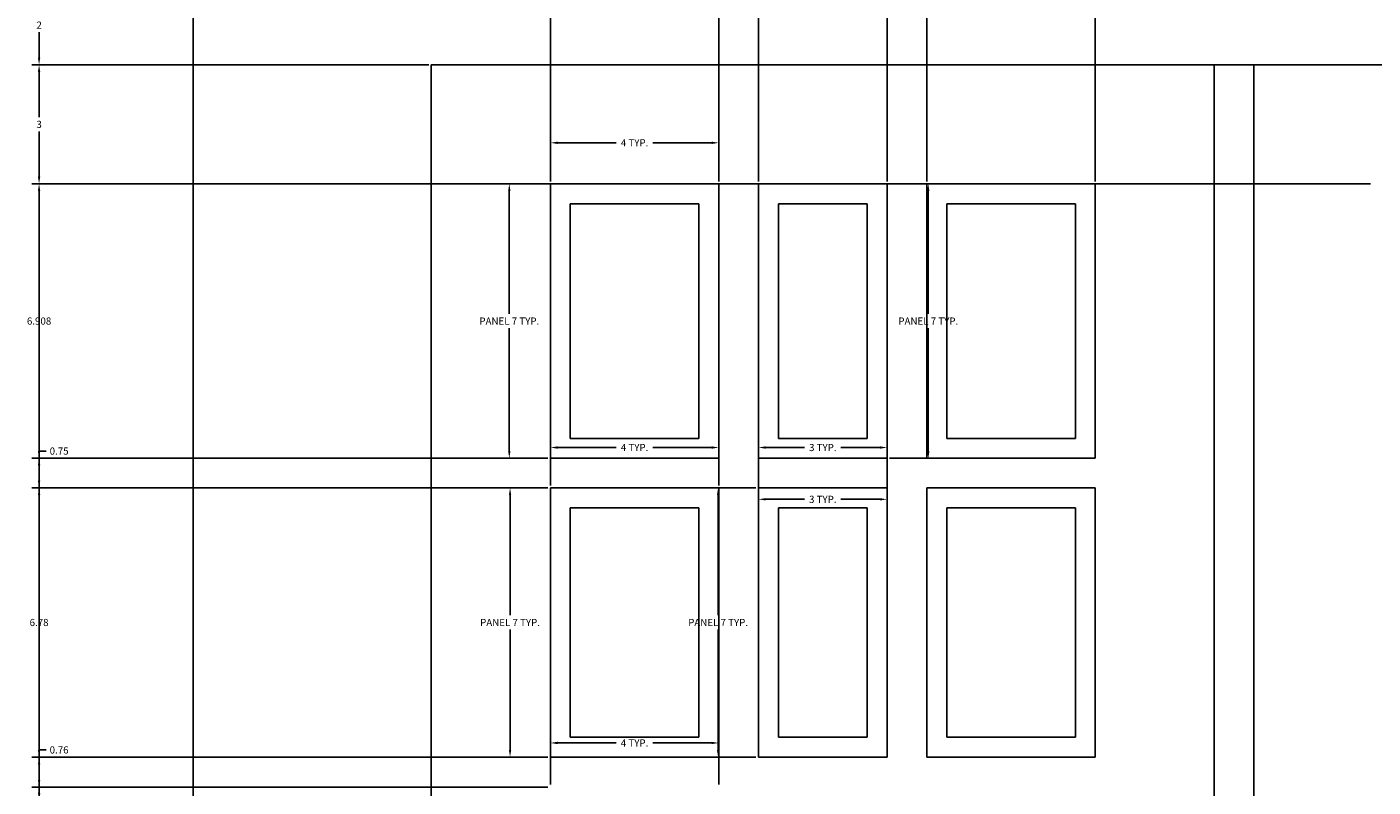
# Model space of a CAD drawing. Units: inches. Extents: x 12532.3 to 12594.9, y 6967.5 to 7063.
# Tile 3 of 9: x 12532.3 to 12566.2, y 7000.7 to 7019.9. Entities that reach past the tile are written whole.
import ezdxf

# ---------------------------------------------------------------- set-up
doc = ezdxf.new("R2010")
doc.units = ezdxf.units.IN
doc.header["$MEASUREMENT"] = 0
doc.header["$PDMODE"] = 98
doc.layers.add('A-ANNO-DIMS', color=2, linetype='Continuous', lineweight=18)
doc.layers.add('A-DOOR', color=4, linetype='Continuous', lineweight=25)
doc.styles.get("Standard").update_dxf_attribs({"font": 'arial.ttf'})
doc.dimstyles.get("Standard").update_dxf_attribs({"dimtxt": 0.18, "dimasz": 0.18, "dimexe": 0.18, "dimexo": 0.0625, "dimgap": 0.09, "dimtad": 0, "dimtih": 1, "dimtoh": 1, "dimdec": 4, "dimzin": 0, "dimdsep": 46, "dimtxsty": 'Standard', "dimcen": 0.09, "dimadec": 0, "dimazin": 0, "dimtfac": 1, "dimtdec": 4, "dimtofl": 0, "dimtmove": 0, "dimatfit": 3, "dimfxl": 1, "dimtolj": 1, "dimtzin": 0, "dimarcsym": 0})

# ---------------------------------------------------------------- blocks, each defined once
blk = doc.blocks.new('DOOR-PANEL-4_2x6_9')
for p, q in [((4.241, 6.908), (0, 6.908)), ((0, 6.908), (0, 0)), ((4.241, 6.908), (4.241, 0)), ((3.741, 6.408), (0.5, 6.408)), ((0.5, 6.408), (0.5, 0.5)), ((3.741, 6.408), (3.741, 0.5)), ((3.741, 0.5), (0.5, 0.5)), ((4.241, 0), (0, 0))]:
    blk.add_line(p, q)
blk = doc.blocks.new('DOOR-PANEL-4_2x6_8')
for p, q in [((4.241, 6.78), (0, 6.78)), ((0, 6.78), (0, 0)), ((4.241, 6.78), (4.241, 0)), ((3.741, 6.28), (0.5, 6.28)), ((0.5, 6.28), (0.5, 0.5)), ((3.741, 6.28), (3.741, 0.5)), ((3.741, 0.5), (0.5, 0.5)), ((4.241, 0), (0, 0))]:
    blk.add_line(p, q)
blk = doc.blocks.new('DOOR-PANEL-3_2x6_8')
for p, q in [((0, 6.78), (0, 0)), ((3.24, 6.78), (0, 6.78)), ((3.24, 6.78), (3.24, 0)), ((0.5, 6.28), (0.5, 0.5)), ((2.74, 6.28), (0.5, 6.28)), ((2.74, 6.28), (2.74, 0.5)), ((2.74, 0.5), (0.5, 0.5)), ((3.24, 0), (0, 0))]:
    blk.add_line(p, q)
blk = doc.blocks.new('DOOR-PANEL-3_2x6_9')
for p, q in [((0, 0), (0, 6.908)), ((0, 6.908), (3.24, 6.908)), ((3.24, 0), (3.24, 6.908)), ((0.5, 0.5), (0.5, 6.408)), ((0.5, 6.408), (2.74, 6.408)), ((2.74, 0.5), (2.74, 6.408)), ((0.5, 0.5), (2.74, 0.5)), ((0, 0), (3.24, 0))]:
    blk.add_line(p, q)
blk = doc.blocks.new('*D13')
at = {"layer": 'A-ANNO-DIMS', "color": 0, "lineweight": -2, "transparency": 16777216}
for p, q in [((12545.388, 7015.929), (12544.234, 7015.929)), ((12544.414, 7015.749), (12544.414, 7012.655)), ((12544.414, 7009.201), (12544.414, 7012.295)), ((12545.388, 7009.021), (12544.234, 7009.021))]:
    blk.add_line(p, q, dxfattribs=at)
at = {"layer": 'A-ANNO-DIMS', "color": 0, "transparency": 16777216}
for points in [[(12544.384, 7015.749), (12544.444, 7015.749), (12544.414, 7015.929)], [(12544.384, 7009.201), (12544.444, 7009.201), (12544.414, 7009.021)]]:
    blk.add_solid(points, dxfattribs=at)
at = {"layer": 'Defpoints', "color": 0, "transparency": 16777216}
for p in [(12545.45, 7015.929), (12544.414, 7009.021), (12545.45, 7009.021)]:
    blk.add_point(p, dxfattribs=at)
at = {"layer": 'A-ANNO-DIMS', "color": 0, "transparency": 16777216, "insert": (12544.414, 7012.475), "char_height": 0.18, "attachment_point": 5}
blk.add_mtext('\\A1;PANEL 7 TYP.', dxfattribs=at)
blk = doc.blocks.new('*D14')
at = {"layer": 'A-ANNO-DIMS', "color": 0, "lineweight": -2, "transparency": 16777216}
for p, q in [((12545.45, 7015.991), (12545.45, 7017.145)), ((12549.691, 7015.991), (12549.691, 7017.145)), ((12545.63, 7016.965), (12547.109, 7016.965)), ((12549.511, 7016.965), (12548.032, 7016.965))]:
    blk.add_line(p, q, dxfattribs=at)
at = {"layer": 'A-ANNO-DIMS', "color": 0, "transparency": 16777216}
for points in [[(12545.63, 7016.995), (12545.63, 7016.935), (12545.45, 7016.965)], [(12549.511, 7016.995), (12549.511, 7016.935), (12549.691, 7016.965)]]:
    blk.add_solid(points, dxfattribs=at)
at = {"layer": 'Defpoints', "color": 0, "transparency": 16777216}
for p in [(12545.45, 7016.965), (12545.45, 7015.929), (12549.691, 7015.929)]:
    blk.add_point(p, dxfattribs=at)
at = {"layer": 'A-ANNO-DIMS', "color": 0, "transparency": 16777216, "insert": (12547.57, 7016.965), "char_height": 0.18, "attachment_point": 5}
blk.add_mtext('\\A1;4 TYP.', dxfattribs=at)
blk = doc.blocks.new('*D15')
at = {"layer": 'A-ANNO-DIMS', "color": 0, "lineweight": -2, "transparency": 16777216}
for p, q in [((12545.388, 7008.273), (12544.253, 7008.273)), ((12544.433, 7008.093), (12544.433, 7005.064)), ((12544.433, 7001.673), (12544.433, 7004.703)), ((12545.388, 7001.493), (12544.253, 7001.493))]:
    blk.add_line(p, q, dxfattribs=at)
at = {"layer": 'A-ANNO-DIMS', "color": 0, "transparency": 16777216}
for points in [[(12544.403, 7008.093), (12544.463, 7008.093), (12544.433, 7008.273)], [(12544.403, 7001.673), (12544.463, 7001.673), (12544.433, 7001.493)]]:
    blk.add_solid(points, dxfattribs=at)
at = {"layer": 'Defpoints', "color": 0, "transparency": 16777216}
for p in [(12545.45, 7008.273), (12544.433, 7001.493), (12545.45, 7001.493)]:
    blk.add_point(p, dxfattribs=at)
at = {"layer": 'A-ANNO-DIMS', "color": 0, "transparency": 16777216, "insert": (12544.433, 7004.883), "char_height": 0.18, "attachment_point": 5}
blk.add_mtext('\\A1;PANEL 7 TYP.', dxfattribs=at)
blk = doc.blocks.new('*D16')
at = {"layer": 'A-ANNO-DIMS', "color": 0, "lineweight": -2, "transparency": 16777216}
for p, q in [((12545.45, 7008.336), (12545.45, 7009.47)), ((12545.63, 7009.29), (12547.109, 7009.29)), ((12549.511, 7009.29), (12548.032, 7009.29)), ((12549.691, 7008.336), (12549.691, 7009.47))]:
    blk.add_line(p, q, dxfattribs=at)
at = {"layer": 'A-ANNO-DIMS', "color": 0, "transparency": 16777216}
for points in [[(12545.63, 7009.32), (12545.63, 7009.26), (12545.45, 7009.29)], [(12549.511, 7009.32), (12549.511, 7009.26), (12549.691, 7009.29)]]:
    blk.add_solid(points, dxfattribs=at)
at = {"layer": 'Defpoints', "color": 0, "transparency": 16777216}
for p in [(12545.45, 7009.29), (12545.45, 7008.273), (12549.691, 7008.273)]:
    blk.add_point(p, dxfattribs=at)
at = {"layer": 'A-ANNO-DIMS', "color": 0, "transparency": 16777216, "insert": (12547.57, 7009.29), "char_height": 0.18, "attachment_point": 5}
blk.add_mtext('\\A1;4 TYP.', dxfattribs=at)
blk = doc.blocks.new('*D18')
at = {"layer": 'A-ANNO-DIMS', "color": 0, "lineweight": -2, "transparency": 16777216}
for p, q in [((12545.45, 7000.8), (12545.45, 7002.029)), ((12545.63, 7001.849), (12547.109, 7001.849)), ((12549.511, 7001.849), (12548.032, 7001.849)), ((12549.691, 7000.8), (12549.691, 7002.029))]:
    blk.add_line(p, q, dxfattribs=at)
at = {"layer": 'A-ANNO-DIMS', "color": 0, "transparency": 16777216}
for points in [[(12545.63, 7001.879), (12545.63, 7001.819), (12545.45, 7001.849)], [(12549.511, 7001.879), (12549.511, 7001.819), (12549.691, 7001.849)]]:
    blk.add_solid(points, dxfattribs=at)
at = {"layer": 'Defpoints', "color": 0, "transparency": 16777216}
for p in [(12545.45, 7001.849), (12545.45, 7000.738), (12549.691, 7000.738)]:
    blk.add_point(p, dxfattribs=at)
at = {"layer": 'A-ANNO-DIMS', "color": 0, "transparency": 16777216, "insert": (12547.57, 7001.849), "char_height": 0.18, "attachment_point": 5}
blk.add_mtext('\\A1;4 TYP.', dxfattribs=at)
blk = doc.blocks.new('*D27')
at = {"layer": 'A-ANNO-DIMS', "color": 0, "lineweight": -2, "transparency": 16777216}
for p, q in [((12550.628, 7008.273), (12549.494, 7008.273)), ((12549.674, 7008.093), (12549.674, 7005.064)), ((12549.674, 7001.673), (12549.674, 7004.703)), ((12550.628, 7001.493), (12549.494, 7001.493))]:
    blk.add_line(p, q, dxfattribs=at)
at = {"layer": 'A-ANNO-DIMS', "color": 0, "transparency": 16777216}
for points in [[(12549.644, 7008.093), (12549.704, 7008.093), (12549.674, 7008.273)], [(12549.644, 7001.673), (12549.704, 7001.673), (12549.674, 7001.493)]]:
    blk.add_solid(points, dxfattribs=at)
at = {"layer": 'Defpoints', "color": 0, "transparency": 16777216}
for p in [(12550.691, 7008.273), (12549.674, 7001.493), (12550.691, 7001.493)]:
    blk.add_point(p, dxfattribs=at)
at = {"layer": 'A-ANNO-DIMS', "color": 0, "transparency": 16777216, "insert": (12549.674, 7004.883), "char_height": 0.18, "attachment_point": 5}
blk.add_mtext('\\A1;PANEL 7 TYP.', dxfattribs=at)
blk = doc.blocks.new('*D28')
at = {"layer": 'A-ANNO-DIMS', "color": 0, "lineweight": -2, "transparency": 16777216}
for p, q in [((12550.691, 7008.336), (12550.691, 7009.47)), ((12550.871, 7009.29), (12551.853, 7009.29)), ((12553.751, 7009.29), (12552.769, 7009.29)), ((12553.931, 7008.336), (12553.931, 7009.47))]:
    blk.add_line(p, q, dxfattribs=at)
at = {"layer": 'A-ANNO-DIMS', "color": 0, "transparency": 16777216}
for points in [[(12550.871, 7009.32), (12550.871, 7009.26), (12550.691, 7009.29)], [(12553.751, 7009.32), (12553.751, 7009.26), (12553.931, 7009.29)]]:
    blk.add_solid(points, dxfattribs=at)
at = {"layer": 'Defpoints', "color": 0, "transparency": 16777216}
for p in [(12550.691, 7009.29), (12550.691, 7008.273), (12553.931, 7008.273)]:
    blk.add_point(p, dxfattribs=at)
at = {"layer": 'A-ANNO-DIMS', "color": 0, "transparency": 16777216, "insert": (12552.311, 7009.29), "char_height": 0.18, "attachment_point": 5}
blk.add_mtext('\\A1;3 TYP.', dxfattribs=at)
blk = doc.blocks.new('*D29')
at = {"layer": 'A-ANNO-DIMS', "color": 0, "lineweight": -2, "transparency": 16777216}
for p, q in [((12553.994, 7015.929), (12555.148, 7015.929)), ((12554.968, 7015.749), (12554.968, 7012.655)), ((12554.968, 7009.201), (12554.968, 7012.295)), ((12553.994, 7009.021), (12555.148, 7009.021))]:
    blk.add_line(p, q, dxfattribs=at)
at = {"layer": 'A-ANNO-DIMS', "color": 0, "transparency": 16777216}
for points in [[(12554.938, 7015.749), (12554.998, 7015.749), (12554.968, 7015.929)], [(12554.938, 7009.201), (12554.998, 7009.201), (12554.968, 7009.021)]]:
    blk.add_solid(points, dxfattribs=at)
at = {"layer": 'Defpoints', "color": 0, "transparency": 16777216}
for p in [(12553.931, 7015.929), (12554.968, 7015.929), (12553.931, 7009.021)]:
    blk.add_point(p, dxfattribs=at)
at = {"layer": 'A-ANNO-DIMS', "color": 0, "transparency": 16777216, "insert": (12554.968, 7012.475), "char_height": 0.18, "attachment_point": 5}
blk.add_mtext('\\A1;PANEL 7 TYP.', dxfattribs=at)
blk = doc.blocks.new('*D30')
at = {"layer": 'A-ANNO-DIMS', "color": 0, "lineweight": -2, "transparency": 16777216}
for p, q in [((12550.691, 7008.959), (12550.691, 7007.805)), ((12553.931, 7008.959), (12553.931, 7007.805)), ((12550.871, 7007.985), (12551.853, 7007.985)), ((12553.751, 7007.985), (12552.769, 7007.985))]:
    blk.add_line(p, q, dxfattribs=at)
at = {"layer": 'A-ANNO-DIMS', "color": 0, "transparency": 16777216}
for points in [[(12550.871, 7008.015), (12550.871, 7007.955), (12550.691, 7007.985)], [(12553.751, 7008.015), (12553.751, 7007.955), (12553.931, 7007.985)]]:
    blk.add_solid(points, dxfattribs=at)
at = {"layer": 'Defpoints', "color": 0, "transparency": 16777216}
for p in [(12550.691, 7009.021), (12553.931, 7009.021), (12553.931, 7007.985)]:
    blk.add_point(p, dxfattribs=at)
at = {"layer": 'A-ANNO-DIMS', "color": 0, "transparency": 16777216, "insert": (12552.311, 7007.985), "char_height": 0.18, "attachment_point": 5}
blk.add_mtext('\\A1;3 TYP.', dxfattribs=at)
blk = doc.blocks.new('*D43')
at = {"layer": 'A-ANNO-DIMS', "color": 0, "lineweight": -2, "transparency": 16777216}
for p, q in [((12566.11, 7015.929), (12532.39, 7015.929)), ((12532.57, 7015.749), (12532.57, 6996.445)), ((12532.57, 6976.777), (12532.57, 6996.081)), ((12566.11, 6976.597), (12532.39, 6976.597))]:
    blk.add_line(p, q, dxfattribs=at)
at = {"layer": 'A-ANNO-DIMS', "color": 0, "transparency": 16777216}
for points in [[(12532.54, 7015.749), (12532.6, 7015.749), (12532.57, 7015.929)], [(12532.54, 6976.777), (12532.6, 6976.777), (12532.57, 6976.597)]]:
    blk.add_solid(points, dxfattribs=at)
at = {"layer": 'Defpoints', "color": 0, "transparency": 16777216}
for p in [(12532.57, 7015.929), (12566.172, 7015.929), (12566.172, 6976.597)]:
    blk.add_point(p, dxfattribs=at)
at = {"layer": 'A-ANNO-DIMS', "color": 0, "transparency": 16777216, "insert": (12532.57, 6996.263), "char_height": 0.18, "attachment_point": 5}
blk.add_mtext('\\A1;39.33', dxfattribs=at)
blk = doc.blocks.new('*D44')
at = {"layer": 'A-ANNO-DIMS', "color": 0, "lineweight": -2, "transparency": 16777216}
for p, q in [((12542.388, 7018.929), (12532.39, 7018.929)), ((12532.57, 7018.749), (12532.57, 7017.611)), ((12532.57, 7016.109), (12532.57, 7017.247)), ((12545.388, 7015.929), (12532.39, 7015.929))]:
    blk.add_line(p, q, dxfattribs=at)
at = {"layer": 'A-ANNO-DIMS', "color": 0, "transparency": 16777216}
for points in [[(12532.54, 7018.749), (12532.6, 7018.749), (12532.57, 7018.929)], [(12532.54, 7016.109), (12532.6, 7016.109), (12532.57, 7015.929)]]:
    blk.add_solid(points, dxfattribs=at)
at = {"layer": 'Defpoints', "color": 0, "transparency": 16777216}
for p in [(12532.57, 7018.929), (12542.45, 7018.929), (12545.45, 7015.929)]:
    blk.add_point(p, dxfattribs=at)
at = {"layer": 'A-ANNO-DIMS', "color": 0, "transparency": 16777216, "insert": (12532.57, 7017.429), "char_height": 0.18, "attachment_point": 5}
blk.add_mtext('\\A1;3', dxfattribs=at)
blk = doc.blocks.new('*D45')
at = {"layer": 'A-ANNO-DIMS', "color": 0, "lineweight": -2, "transparency": 16777216}
for p, q in [((12536.388, 7020.929), (12532.39, 7020.929)), ((12532.57, 7020.749), (12532.57, 7020.109)), ((12532.57, 7019.109), (12532.57, 7019.748)), ((12542.388, 7018.929), (12532.39, 7018.929))]:
    blk.add_line(p, q, dxfattribs=at)
at = {"layer": 'A-ANNO-DIMS', "color": 0, "transparency": 16777216}
for points in [[(12532.54, 7020.749), (12532.6, 7020.749), (12532.57, 7020.929)], [(12532.54, 7019.109), (12532.6, 7019.109), (12532.57, 7018.929)]]:
    blk.add_solid(points, dxfattribs=at)
at = {"layer": 'Defpoints', "color": 0, "transparency": 16777216}
for p in [(12532.57, 7020.929), (12536.45, 7020.929), (12542.45, 7018.929)]:
    blk.add_point(p, dxfattribs=at)
at = {"layer": 'A-ANNO-DIMS', "color": 0, "transparency": 16777216, "insert": (12532.57, 7019.929), "char_height": 0.18, "attachment_point": 5}
blk.add_mtext('\\A1;2', dxfattribs=at)
blk = doc.blocks.new('*D46')
at = {"layer": 'A-ANNO-DIMS', "color": 0, "lineweight": -2, "transparency": 16777216}
for p, q in [((12545.45, 7015.991), (12545.45, 7051.211)), ((12545.63, 7051.031), (12547.191, 7051.031)), ((12549.511, 7051.031), (12547.95, 7051.031)), ((12549.691, 7015.991), (12549.691, 7051.211))]:
    blk.add_line(p, q, dxfattribs=at)
at = {"layer": 'A-ANNO-DIMS', "color": 0, "transparency": 16777216}
for points in [[(12545.63, 7051.061), (12545.63, 7051.001), (12545.45, 7051.031)], [(12549.511, 7051.061), (12549.511, 7051.001), (12549.691, 7051.031)]]:
    blk.add_solid(points, dxfattribs=at)
at = {"layer": 'Defpoints', "color": 0, "transparency": 16777216}
for p in [(12549.691, 7051.031), (12545.45, 7015.929), (12549.691, 7015.929)]:
    blk.add_point(p, dxfattribs=at)
at = {"layer": 'A-ANNO-DIMS', "color": 0, "transparency": 16777216, "insert": (12547.57, 7051.031), "char_height": 0.18, "attachment_point": 5}
blk.add_mtext('\\A1;4.241', dxfattribs=at)
blk = doc.blocks.new('*D47')
at = {"layer": 'A-ANNO-DIMS', "color": 0, "lineweight": -2, "transparency": 16777216}
for p, q in [((12549.691, 7015.991), (12549.691, 7051.211)), ((12549.871, 7051.031), (12550.068, 7051.031)), ((12550.511, 7051.031), (12550.314, 7051.031)), ((12550.691, 7015.991), (12550.691, 7051.211))]:
    blk.add_line(p, q, dxfattribs=at)
at = {"layer": 'A-ANNO-DIMS', "color": 0, "transparency": 16777216}
for points in [[(12549.871, 7051.061), (12549.871, 7051.001), (12549.691, 7051.031)], [(12550.511, 7051.061), (12550.511, 7051.001), (12550.691, 7051.031)]]:
    blk.add_solid(points, dxfattribs=at)
at = {"layer": 'Defpoints', "color": 0, "transparency": 16777216}
for p in [(12550.691, 7051.031), (12549.691, 7015.929), (12550.691, 7015.929)]:
    blk.add_point(p, dxfattribs=at)
at = {"layer": 'A-ANNO-DIMS', "color": 0, "transparency": 16777216, "insert": (12550.191, 7051.031), "char_height": 0.18, "attachment_point": 5}
blk.add_mtext('\\A1;1', dxfattribs=at)
blk = doc.blocks.new('*D48')
at = {"layer": 'A-ANNO-DIMS', "color": 0, "lineweight": -2, "transparency": 16777216}
for p, q in [((12550.691, 7015.991), (12550.691, 7051.211)), ((12550.871, 7051.031), (12551.988, 7051.031)), ((12553.751, 7051.031), (12552.634, 7051.031)), ((12553.931, 7015.991), (12553.931, 7051.211))]:
    blk.add_line(p, q, dxfattribs=at)
at = {"layer": 'A-ANNO-DIMS', "color": 0, "transparency": 16777216}
for points in [[(12550.871, 7051.061), (12550.871, 7051.001), (12550.691, 7051.031)], [(12553.751, 7051.061), (12553.751, 7051.001), (12553.931, 7051.031)]]:
    blk.add_solid(points, dxfattribs=at)
at = {"layer": 'Defpoints', "color": 0, "transparency": 16777216}
for p in [(12553.931, 7051.031), (12550.691, 7015.929), (12553.931, 7015.929)]:
    blk.add_point(p, dxfattribs=at)
at = {"layer": 'A-ANNO-DIMS', "color": 0, "transparency": 16777216, "insert": (12552.311, 7051.031), "char_height": 0.18, "attachment_point": 5}
blk.add_mtext('\\A1;3.24', dxfattribs=at)
blk = doc.blocks.new('*D49')
at = {"layer": 'A-ANNO-DIMS', "color": 0, "lineweight": -2, "transparency": 16777216}
for p, q in [((12553.931, 7015.991), (12553.931, 7051.211)), ((12554.111, 7051.031), (12554.308, 7051.031)), ((12554.751, 7051.031), (12554.555, 7051.031)), ((12554.931, 7015.991), (12554.931, 7051.211))]:
    blk.add_line(p, q, dxfattribs=at)
at = {"layer": 'A-ANNO-DIMS', "color": 0, "transparency": 16777216}
for points in [[(12554.111, 7051.061), (12554.111, 7051.001), (12553.931, 7051.031)], [(12554.751, 7051.061), (12554.751, 7051.001), (12554.931, 7051.031)]]:
    blk.add_solid(points, dxfattribs=at)
at = {"layer": 'Defpoints', "color": 0, "transparency": 16777216}
for p in [(12554.931, 7051.031), (12553.931, 7015.929), (12554.931, 7015.929)]:
    blk.add_point(p, dxfattribs=at)
at = {"layer": 'A-ANNO-DIMS', "color": 0, "transparency": 16777216, "insert": (12554.431, 7051.031), "char_height": 0.18, "attachment_point": 5}
blk.add_mtext('\\A1;1', dxfattribs=at)
blk = doc.blocks.new('*D50')
at = {"layer": 'A-ANNO-DIMS', "color": 0, "lineweight": -2, "transparency": 16777216}
for p, q in [((12554.931, 7015.991), (12554.931, 7051.211)), ((12555.111, 7051.031), (12556.672, 7051.031)), ((12558.992, 7051.031), (12557.432, 7051.031)), ((12559.172, 7015.991), (12559.172, 7051.211))]:
    blk.add_line(p, q, dxfattribs=at)
at = {"layer": 'A-ANNO-DIMS', "color": 0, "transparency": 16777216}
for points in [[(12555.111, 7051.061), (12555.111, 7051.001), (12554.931, 7051.031)], [(12558.992, 7051.061), (12558.992, 7051.001), (12559.172, 7051.031)]]:
    blk.add_solid(points, dxfattribs=at)
at = {"layer": 'Defpoints', "color": 0, "transparency": 16777216}
for p in [(12559.172, 7051.031), (12554.931, 7015.929), (12559.172, 7015.929)]:
    blk.add_point(p, dxfattribs=at)
at = {"layer": 'A-ANNO-DIMS', "color": 0, "transparency": 16777216, "insert": (12557.052, 7051.031), "char_height": 0.18, "attachment_point": 5}
blk.add_mtext('\\A1;4.241', dxfattribs=at)
blk = doc.blocks.new('*D55')
at = {"layer": 'A-ANNO-DIMS', "color": 0, "lineweight": -2, "transparency": 16777216}
for p, q in [((12545.388, 7000.738), (12532.39, 7000.738)), ((12532.57, 7000.558), (12532.57, 6997.216)), ((12532.57, 6993.51), (12532.57, 6996.852)), ((12545.388, 6993.33), (12532.39, 6993.33))]:
    blk.add_line(p, q, dxfattribs=at)
at = {"layer": 'A-ANNO-DIMS', "color": 0, "transparency": 16777216}
for points in [[(12532.54, 7000.558), (12532.6, 7000.558), (12532.57, 7000.738)], [(12532.54, 6993.51), (12532.6, 6993.51), (12532.57, 6993.33)]]:
    blk.add_solid(points, dxfattribs=at)
at = {"layer": 'Defpoints', "color": 0, "transparency": 16777216}
for p in [(12532.57, 7000.738), (12545.45, 7000.738), (12545.45, 6993.33)]:
    blk.add_point(p, dxfattribs=at)
at = {"layer": 'A-ANNO-DIMS', "color": 0, "transparency": 16777216, "insert": (12532.57, 6997.034), "char_height": 0.18, "attachment_point": 5}
blk.add_mtext('\\A1;7.407', dxfattribs=at)
blk = doc.blocks.new('*D56')
at = {"layer": 'A-ANNO-DIMS', "color": 0, "lineweight": -2, "transparency": 16777216}
for p, q in [((12545.388, 7001.493), (12532.39, 7001.493)), ((12532.57, 7001.493), (12532.57, 7001.673)), ((12532.57, 7001.673), (12532.75, 7001.673)), ((12532.57, 7000.918), (12532.57, 7001.313)), ((12545.388, 7000.738), (12532.39, 7000.738))]:
    blk.add_line(p, q, dxfattribs=at)
at = {"layer": 'A-ANNO-DIMS', "color": 0, "transparency": 16777216}
for points in [[(12532.54, 7001.313), (12532.6, 7001.313), (12532.57, 7001.493)], [(12532.54, 7000.918), (12532.6, 7000.918), (12532.57, 7000.738)]]:
    blk.add_solid(points, dxfattribs=at)
at = {"layer": 'Defpoints', "color": 0, "transparency": 16777216}
for p in [(12532.57, 7001.493), (12545.45, 7001.493), (12545.45, 7000.738)]:
    blk.add_point(p, dxfattribs=at)
at = {"layer": 'A-ANNO-DIMS', "color": 0, "transparency": 16777216, "insert": (12533.074, 7001.673), "char_height": 0.18, "attachment_point": 5}
blk.add_mtext('\\A1;0.76', dxfattribs=at)
blk = doc.blocks.new('*D57')
at = {"layer": 'A-ANNO-DIMS', "color": 0, "lineweight": -2, "transparency": 16777216}
for p, q in [((12545.388, 7008.273), (12532.39, 7008.273)), ((12532.57, 7008.093), (12532.57, 7005.065)), ((12532.57, 7001.673), (12532.57, 7004.702)), ((12545.388, 7001.493), (12532.39, 7001.493))]:
    blk.add_line(p, q, dxfattribs=at)
at = {"layer": 'A-ANNO-DIMS', "color": 0, "transparency": 16777216}
for points in [[(12532.54, 7008.093), (12532.6, 7008.093), (12532.57, 7008.273)], [(12532.54, 7001.673), (12532.6, 7001.673), (12532.57, 7001.493)]]:
    blk.add_solid(points, dxfattribs=at)
at = {"layer": 'Defpoints', "color": 0, "transparency": 16777216}
for p in [(12532.57, 7008.273), (12545.45, 7008.273), (12545.45, 7001.493)]:
    blk.add_point(p, dxfattribs=at)
at = {"layer": 'A-ANNO-DIMS', "color": 0, "transparency": 16777216, "insert": (12532.57, 7004.883), "char_height": 0.18, "attachment_point": 5}
blk.add_mtext('\\A1;6.78', dxfattribs=at)
blk = doc.blocks.new('*D58')
at = {"layer": 'A-ANNO-DIMS', "color": 0, "lineweight": -2, "transparency": 16777216}
for p, q in [((12545.388, 7009.021), (12532.39, 7009.021)), ((12532.57, 7009.021), (12532.57, 7009.201)), ((12532.57, 7009.201), (12532.75, 7009.201)), ((12532.57, 7008.453), (12532.57, 7008.841)), ((12545.388, 7008.273), (12532.39, 7008.273))]:
    blk.add_line(p, q, dxfattribs=at)
at = {"layer": 'A-ANNO-DIMS', "color": 0, "transparency": 16777216}
for points in [[(12532.54, 7008.841), (12532.6, 7008.841), (12532.57, 7009.021)], [(12532.54, 7008.453), (12532.6, 7008.453), (12532.57, 7008.273)]]:
    blk.add_solid(points, dxfattribs=at)
at = {"layer": 'Defpoints', "color": 0, "transparency": 16777216}
for p in [(12532.57, 7009.021), (12545.45, 7009.021), (12545.45, 7008.273)]:
    blk.add_point(p, dxfattribs=at)
at = {"layer": 'A-ANNO-DIMS', "color": 0, "transparency": 16777216, "insert": (12533.075, 7009.201), "char_height": 0.18, "attachment_point": 5}
blk.add_mtext('\\A1;0.75', dxfattribs=at)
blk = doc.blocks.new('*D59')
at = {"layer": 'A-ANNO-DIMS', "color": 0, "lineweight": -2, "transparency": 16777216}
for p, q in [((12545.388, 7015.929), (12532.39, 7015.929)), ((12532.57, 7015.749), (12532.57, 7012.657)), ((12532.57, 7009.201), (12532.57, 7012.293)), ((12545.388, 7009.021), (12532.39, 7009.021))]:
    blk.add_line(p, q, dxfattribs=at)
at = {"layer": 'A-ANNO-DIMS', "color": 0, "transparency": 16777216}
for points in [[(12532.54, 7015.749), (12532.6, 7015.749), (12532.57, 7015.929)], [(12532.54, 7009.201), (12532.6, 7009.201), (12532.57, 7009.021)]]:
    blk.add_solid(points, dxfattribs=at)
at = {"layer": 'Defpoints', "color": 0, "transparency": 16777216}
for p in [(12532.57, 7015.929), (12545.45, 7015.929), (12545.45, 7009.021)]:
    blk.add_point(p, dxfattribs=at)
at = {"layer": 'A-ANNO-DIMS', "color": 0, "transparency": 16777216, "insert": (12532.57, 7012.475), "char_height": 0.18, "attachment_point": 5}
blk.add_mtext('\\A1;6.908', dxfattribs=at)

msp = doc.modelspace()

# ---------------------------------------------------------------- linework, layer by layer
at = {"layer": 'A-DOOR'}
for p, q in [((12562.1721, 6973.5968), (12562.1721, 7018.9287)), ((12563.1721, 6973.5968), (12563.1721, 7018.9287))]:
    msp.add_line(p, q, dxfattribs=at)
msp.add_lwpolyline([(12536.4501, 7020.9287), (12588.894, 7020.9287), (12588.894, 6971.5968), (12536.4501, 6971.5968)], close=True, dxfattribs=at)
for points in [[(12542.4501, 7018.9287), (12582.894, 7018.9287)], [(12542.4501, 6973.5968), (12542.4501, 7018.9287)]]:
    msp.add_lwpolyline(points, dxfattribs=at)

# ---------------------------------------------------------------- block references
at = {"layer": 'A-DOOR', "rotation": 180}
for name, p in [('DOOR-PANEL-4_2x6_9', (12549.6909, 7015.9287)), ('DOOR-PANEL-4_2x6_8', (12549.6909, 7008.2739)), ('DOOR-PANEL-3_2x6_8', (12553.9312, 7008.2739))]:
    msp.add_blockref(name, p, dxfattribs=at)
at = {"layer": 'A-DOOR'}
for name, p in [('DOOR-PANEL-3_2x6_9', (12550.691, 7009.021)), ('DOOR-PANEL-4_2x6_9', (12554.9313, 7009.021)), ('DOOR-PANEL-4_2x6_8', (12554.9313, 7001.493))]:
    msp.add_blockref(name, p, dxfattribs=at)

# ---------------------------------------------------------------- dimensions: what is measured, and where the dimension line sits
at = {"layer": 'A-ANNO-DIMS'}
for base, p1, p2, override, picture, middle in [((12549.6908, 7051.0306), (12545.4501, 7015.9287), (12549.6908, 7015.9287), {"dimdec": 3, "dimlfac": 1, "dimrnd": 0, "dimzin": 0, "dimdsep": 46, "dimlunit": 2}, '*D46', (12547.5705, 7051.0306)), ((12550.6908, 7051.0306), (12549.6908, 7015.9287), (12550.6908, 7015.9287), {"dimdec": 0, "dimlfac": 1, "dimrnd": 0, "dimzin": 0, "dimdsep": 46, "dimlunit": 2}, '*D47', (12550.1908, 7051.0306)), ((12553.9314, 7051.0306), (12550.6908, 7015.9287), (12553.9314, 7015.9287), {"dimdec": 2, "dimlfac": 1, "dimrnd": 0, "dimzin": 0, "dimdsep": 46, "dimlunit": 2}, '*D48', (12552.3111, 7051.0306)), ((12554.9314, 7051.0306), (12553.9314, 7015.9287), (12554.9314, 7015.9287), {"dimdec": 0, "dimlfac": 1, "dimrnd": 0, "dimzin": 0, "dimdsep": 46, "dimlunit": 2}, '*D49', (12554.4314, 7051.0306)), ((12559.1721, 7051.0306), (12554.9314, 7015.9287), (12559.1721, 7015.9287), {"dimdec": 3, "dimlfac": 1, "dimrnd": 0, "dimzin": 0, "dimdsep": 46, "dimlunit": 2}, '*D50', (12557.0518, 7051.0306))]:
    dim = msp.add_linear_dim(base=base, p1=p1, p2=p2, dimstyle='Standard', override=override, dxfattribs=at)
    dim.commit()
    dim.dimension.update_dxf_attribs({"geometry": picture, "text_midpoint": middle})
for base, p1, p2, override, picture, middle in [((12532.5701, 7020.9287), (12542.4501, 7018.9287), (12536.4501, 7020.9287), {"dimdec": 0, "dimlfac": 1, "dimrnd": 0, "dimzin": 0, "dimdsep": 46, "dimlunit": 2}, '*D45', (12532.5701, 7019.9287)), ((12532.5701, 7018.9287), (12545.4501, 7015.9287), (12542.4501, 7018.9287), {"dimdec": 0, "dimlfac": 1, "dimrnd": 0, "dimzin": 0, "dimdsep": 46, "dimlunit": 2}, '*D44', (12532.5701, 7017.4287)), ((12532.5701, 7015.9287), (12566.1721, 6976.5968), (12566.1721, 7015.9287), {"dimdec": 2, "dimlfac": 1, "dimrnd": 0, "dimzin": 0, "dimdsep": 46, "dimlunit": 2}, '*D43', (12532.5701, 6996.2627)), ((12532.5701, 7015.9287), (12545.4501, 7009.021), (12545.4501, 7015.9287), {"dimdec": 3, "dimlfac": 1, "dimrnd": 0, "dimzin": 0, "dimdsep": 46, "dimlunit": 2}, '*D59', (12532.5701, 7012.4749)), ((12532.5701, 7009.021), (12545.4501, 7008.2735), (12545.4501, 7009.021), {"dimdec": 2, "dimlfac": 1, "dimrnd": 0, "dimzin": 0, "dimdsep": 46, "dimlunit": 2}, '*D58', (12533.0746, 7009.201)), ((12532.5701, 7008.2735), (12545.4501, 7001.4934), (12545.4501, 7008.2735), {"dimdec": 2, "dimlfac": 1, "dimrnd": 0, "dimzin": 0, "dimdsep": 46, "dimlunit": 2}, '*D57', (12532.5701, 7004.8834)), ((12532.5701, 7001.4934), (12545.4501, 7000.7376), (12545.4501, 7001.4934), {"dimdec": 2, "dimlfac": 1, "dimrnd": 0, "dimzin": 0, "dimdsep": 46, "dimlunit": 2}, '*D56', (12533.0739, 7001.6734)), ((12532.5701, 7000.7376), (12545.4501, 6993.3303), (12545.4501, 7000.7376), {"dimdec": 3, "dimlfac": 1, "dimrnd": 0, "dimzin": 0, "dimdsep": 46, "dimlunit": 2}, '*D55', (12532.5701, 6997.034))]:
    dim = msp.add_linear_dim(base=base, p1=p1, p2=p2, angle=90, dimstyle='Standard', override=override, dxfattribs=at)
    dim.commit()
    dim.dimension.update_dxf_attribs({"geometry": picture, "text_midpoint": middle})
for base, p1, p2, angle, text, picture, middle in [((12545.4501, 7016.9649), (12549.6908, 7015.9287), (12545.4501, 7015.9287), 180, '<> TYP.', '*D14', (12547.5705, 7016.9649)), ((12544.414, 7009.021), (12545.4501, 7015.9287), (12545.4501, 7009.021), 270, 'PANEL <> TYP.', '*D13', (12544.414, 7012.4749)), ((12554.9676, 7015.9287), (12553.9314, 7009.021), (12553.9314, 7015.9287), 90, 'PANEL <> TYP.', '*D29', (12554.9676, 7012.4749)), ((12545.4501, 7009.2905), (12549.6908, 7008.2735), (12545.4501, 7008.2735), 180, '<> TYP.', '*D16', (12547.5705, 7009.2905)), ((12550.6908, 7009.2905), (12553.9314, 7008.2735), (12550.6908, 7008.2735), 180, '<> TYP.', '*D28', (12552.3111, 7009.2905)), ((12544.4331, 7001.4934), (12545.4501, 7008.2735), (12545.4501, 7001.4934), 270, 'PANEL <> TYP.', '*D15', (12544.4331, 7004.8834)), ((12549.6738, 7001.4934), (12550.6908, 7008.2735), (12550.6908, 7001.4934), 270, 'PANEL <> TYP.', '*D27', (12549.6738, 7004.8834)), ((12545.4501, 7001.8487), (12549.6908, 7000.7376), (12545.4501, 7000.7376), 180, '<> TYP.', '*D18', (12547.5705, 7001.8487))]:
    dim = msp.add_linear_dim(base=base, p1=p1, p2=p2, angle=angle, text=text, dimstyle='Standard', override={"dimdec": 0, "dimrnd": 0, "dimzin": 0, "dimlunit": 2}, dxfattribs=at)
    dim.commit()
    dim.dimension.update_dxf_attribs({"geometry": picture, "text_midpoint": middle})
dim = msp.add_linear_dim(base=(12553.9314, 7007.9848), p1=(12550.6908, 7009.021), p2=(12553.9314, 7009.021), text='<> TYP.', dimstyle='Standard', override={"dimdec": 0, "dimrnd": 0, "dimzin": 0, "dimlunit": 2}, dxfattribs=at)
dim.commit()
dim.dimension.update_dxf_attribs({"geometry": '*D30', "text_midpoint": (12552.3111, 7007.9848)})

doc.saveas('drawing.dxf')
